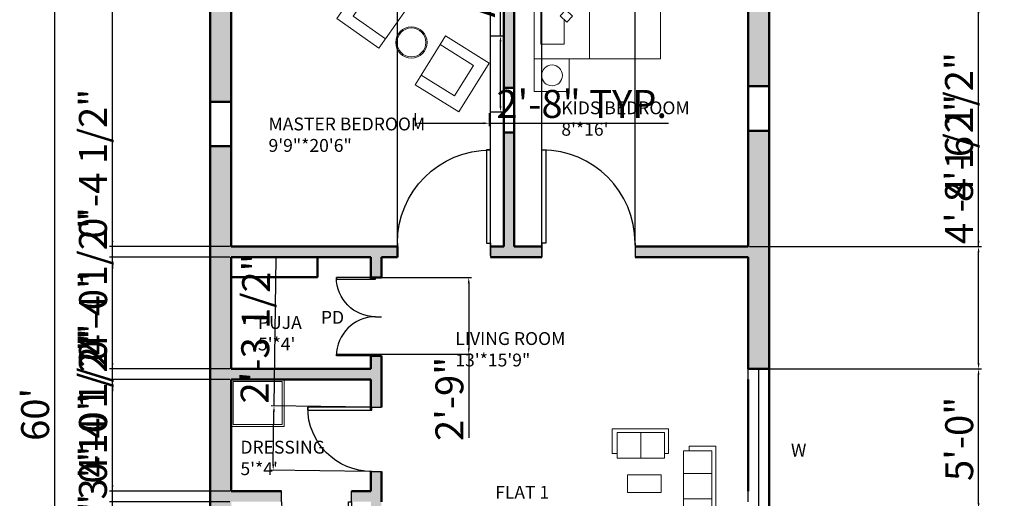
# Model space of a CAD drawing. Units: inches. Extents: x 2063 to 3370, y 2091 to 2971.
# Tile 6 of 14: x 2063 to 2486, y 2468 to 2674. Entities that reach past the tile are written whole.
import ezdxf

# ---------------------------------------------------------------- set-up
doc = ezdxf.new("R2010")
doc.units = ezdxf.units.IN
for name, color, linetype, lineweight in [('A-ANNO-DIMS', 2, 'Continuous', 18), ('A-ANNO-TEXT', 7, 'Continuous', 18), ('A-AREA-IDEN', 3, 'Continuous', 18), ('A-COLS', 7, 'Continuous', 50), ('A-DOOR', 4, 'Continuous', 25), ('A-FURN', 8, 'Continuous', 18), ('A-GLAZ', 131, 'Continuous', 25), ('A-WALL', 7, 'Continuous', 50), ('A-WALL-PATT', 8, 'Continuous', 13)]:
    doc.layers.add(name, color=color, linetype=linetype, lineweight=lineweight)
doc.styles.get("Standard").update_dxf_attribs({"font": 'arial.ttf'})
doc.dimstyles.new('ISO-25', dxfattribs={"dimtxt": 12, "dimasz": 2.5, "dimexe": 1.25, "dimexo": 0.625, "dimtad": 1, "dimdec": 0, "dimlunit": 4, "dimtxsty": 'Standard', "dimcen": 2.5, "dimadec": 0, "dimazin": 0, "dimtfac": 1, "dimtdec": 0, "dimtmove": 0, "dimatfit": 3, "dimfxl": 1, "dimarcsym": 0})

# ---------------------------------------------------------------- blocks, each defined once
blk = doc.blocks.new('*U2')
for p, q in [((0, 0), (0, -6)), ((40, 0), (40, -6))]:
    blk.add_line(p, q)
blk.add_lwpolyline([(0, 0), (0, 40), (1.75, 40), (1.75, 0)], close=True)
blk.add_arc((0, 0), 40, 0, 90)
blk = doc.blocks.new('*D6')
at = {"layer": 'A-ANNO-DIMS', "color": 0, "lineweight": -2, "transparency": 16777216}
for p, q in [((2144.1, 2864.43), (2076.56, 2864.43)), ((2077.81, 2861.93), (2077.81, 2146.93)), ((2144.1, 2144.43), (2076.56, 2144.43))]:
    blk.add_line(p, q, dxfattribs=at)
at = {"layer": 'A-ANNO-DIMS', "color": 0, "transparency": 16777216}
for points in [[(2077.39, 2861.93), (2078.23, 2861.93), (2077.81, 2864.43)], [(2077.39, 2146.93), (2078.23, 2146.93), (2077.81, 2144.43)]]:
    blk.add_solid(points, dxfattribs=at)
at = {"layer": 'Defpoints', "color": 0, "transparency": 16777216}
for p in [(2144.72, 2864.43), (2077.81, 2144.43), (2144.72, 2144.43)]:
    blk.add_point(p, dxfattribs=at)
at = {"layer": 'A-ANNO-DIMS', "color": 0, "transparency": 16777216, "insert": (2071.06, 2504.43), "char_height": 12, "attachment_point": 5, "rotation": 90}
blk.add_mtext("60'", dxfattribs=at)
blk = doc.blocks.new('BED-DOUBLE')
for p, q in [((23.79, 50.98), (30.96, 58.78)), ((30.96, 58.78), (30.96, 50.54)), ((23.79, 14), (23.79, 50.98)), ((30.96, 50.54), (23.79, 50.98))]:
    blk.add_line(p, q)
for points in [[(0, 58.78), (15.11, 58.78), (15.11, 72.78), (0, 72.78)], [(0, 58.78), (54.26, 58.78), (54.26, 14), (0, 14)], [(11.45, 40.86), (13.89, 43.46), (16.84, 40.71), (14.4, 38.1)], [(11.16, 32.43), (13.59, 35.03), (16.54, 32.28), (14.11, 29.67)], [(0, 0), (15.11, 0), (15.11, 14), (0, 14)]]:
    blk.add_lwpolyline(points, close=True)
for points in [[(12.88, 42.39), (12.88, 53.87), (2.9, 53.87), (2.9, 35.71), (12.88, 35.71), (12.88, 39.52)], [(12.88, 34.27), (12.88, 38.39), (2.9, 38.39), (2.9, 20.23), (12.88, 20.23), (12.88, 30.81)]]:
    blk.add_lwpolyline(points)
for centre, radius in [((7.71, 65.74), 4.47), ((15.81, 36.46), 1.81), ((7.71, 6.86), 4.47)]:
    blk.add_circle(centre, radius)
blk = doc.blocks.new('ARMCHAIR')
for p, q in [((10.7, 28.87), (13.03, 32.61)), ((13.03, 32.61), (31.78, 20.96)), ((0, 11.65), (3.54, 17.35)), ((31.78, 20.96), (18.75, 0)), ((18.75, 0), (0, 11.65))]:
    blk.add_line(p, q)
blk.add_lwpolyline([(2.55, 15.75), (16.92, 6.82), (25.07, 19.93), (10.7, 28.87)], close=True)
blk = doc.blocks.new('SOFA-2SEAT')
for p, q in [((0, 2.07), (0, 12.63)), ((0, 12.63), (24.16, 12.63)), ((12.27, 11.03), (12.27, 0)), ((24.16, 12.63), (24.16, 2.07)), ((2.08, 2.07), (0, 2.07)), ((24.16, 2.07), (22.46, 2.07))]:
    blk.add_line(p, q)
blk.add_lwpolyline([(22.46, 0), (2.08, 0), (2.08, 11.03), (22.46, 11.03)], close=True)
blk = doc.blocks.new('SOFA-3SEAT')
for p, q in [((2.4, 33.13), (2.4, 35.12)), ((2.4, 35.12), (13.91, 35.12)), ((13.91, 35.12), (13.91, 0)), ((0, 23.31), (12.18, 23.31)), ((0, 12.42), (12.18, 12.42)), ((2.4, 0), (2.4, 1.81)), ((13.91, 0), (2.4, 0))]:
    blk.add_line(p, q)
blk.add_lwpolyline([(12.18, 33.13), (0, 33.13), (0, 1.81), (12.18, 1.81)], close=True)
blk = doc.blocks.new('*D24')
at = {"layer": 'A-ANNO-DIMS', "color": 0, "lineweight": -2, "transparency": 16777216}
for p, q in [((2269.34, 2666.87), (2269.34, 2866.5)), ((2265.08, 2666.87), (2270.59, 2666.87)), ((2269.34, 2636.76), (2269.34, 2664.37)), ((2265.08, 2634.26), (2270.59, 2634.26))]:
    blk.add_line(p, q, dxfattribs=at)
at = {"layer": 'A-ANNO-DIMS', "color": 0, "transparency": 16777216}
for points in [[(2268.93, 2664.37), (2269.76, 2664.37), (2269.34, 2666.87)], [(2268.93, 2636.76), (2269.76, 2636.76), (2269.34, 2634.26)]]:
    blk.add_solid(points, dxfattribs=at)
at = {"layer": 'Defpoints', "color": 0, "transparency": 16777216}
for p in [(2264.45, 2666.87), (2269.34, 2666.87), (2264.45, 2634.26)]:
    blk.add_point(p, dxfattribs=at)
at = {"layer": 'A-ANNO-DIMS', "color": 0, "transparency": 16777216, "insert": (2262.51, 2767.94), "char_height": 12, "attachment_point": 5, "rotation": 90}
blk.add_mtext('ARMCHAIR 2\'-8 1/2" TYP.', dxfattribs=at)
blk = doc.blocks.new('*D25')
at = {"layer": 'A-ANNO-DIMS', "color": 0, "lineweight": -2, "transparency": 16777216}
for p, q in [((2232.68, 2633.64), (2232.68, 2628.12)), ((2264.45, 2633.64), (2264.45, 2628.12)), ((2235.18, 2629.37), (2261.95, 2629.37)), ((2264.45, 2629.37), (2341.55, 2629.37))]:
    blk.add_line(p, q, dxfattribs=at)
at = {"layer": 'A-ANNO-DIMS', "color": 0, "transparency": 16777216}
for points in [[(2235.18, 2629.79), (2235.18, 2628.95), (2232.68, 2629.37)], [(2261.95, 2629.79), (2261.95, 2628.95), (2264.45, 2629.37)]]:
    blk.add_solid(points, dxfattribs=at)
at = {"layer": 'Defpoints', "color": 0, "transparency": 16777216}
for p in [(2232.68, 2634.26), (2264.45, 2634.26), (2264.45, 2629.37)]:
    blk.add_point(p, dxfattribs=at)
at = {"layer": 'A-ANNO-DIMS', "color": 0, "transparency": 16777216, "insert": (2304.25, 2636.12), "char_height": 12, "attachment_point": 5}
blk.add_mtext('2\'-8" TYP.', dxfattribs=at)
blk = doc.blocks.new('*D50')
at = {"layer": 'A-ANNO-DIMS', "color": 0, "lineweight": -2, "transparency": 16777216}
for p, q in [((2102.72, 2396.38), (2102.72, 2468.18)), ((2153.1, 2396.38), (2101.47, 2396.38)), ((2102.72, 2376.43), (2102.72, 2393.88)), ((2153.1, 2373.93), (2101.47, 2373.93))]:
    blk.add_line(p, q, dxfattribs=at)
at = {"layer": 'A-ANNO-DIMS', "color": 0, "transparency": 16777216}
for points in [[(2102.31, 2393.88), (2103.14, 2393.88), (2102.72, 2396.38)], [(2102.31, 2376.43), (2103.14, 2376.43), (2102.72, 2373.93)]]:
    blk.add_solid(points, dxfattribs=at)
at = {"layer": 'Defpoints', "color": 0, "transparency": 16777216}
for p in [(2102.72, 2396.38), (2153.72, 2396.38), (2153.72, 2373.93)]:
    blk.add_point(p, dxfattribs=at)
at = {"layer": 'A-ANNO-DIMS', "color": 0, "transparency": 16777216, "insert": (2095.89, 2433.53), "char_height": 12, "attachment_point": 5, "rotation": 90}
blk.add_mtext('1\'-10 1/2"', dxfattribs=at)
blk = doc.blocks.new('*D52')
at = {"layer": 'A-ANNO-DIMS', "color": 0, "lineweight": -2, "transparency": 16777216}
for p, q in [((2102.72, 2466.93), (2102.72, 2539.85)), ((2153.1, 2466.93), (2101.47, 2466.93)), ((2102.72, 2422.88), (2102.72, 2464.43)), ((2153.1, 2420.38), (2101.47, 2420.38))]:
    blk.add_line(p, q, dxfattribs=at)
at = {"layer": 'A-ANNO-DIMS', "color": 0, "transparency": 16777216}
for points in [[(2102.31, 2464.43), (2103.14, 2464.43), (2102.72, 2466.93)], [(2102.31, 2422.88), (2103.14, 2422.88), (2102.72, 2420.38)]]:
    blk.add_solid(points, dxfattribs=at)
at = {"layer": 'Defpoints', "color": 0, "transparency": 16777216}
for p in [(2102.72, 2466.93), (2153.72, 2466.93), (2153.72, 2420.38)]:
    blk.add_point(p, dxfattribs=at)
at = {"layer": 'A-ANNO-DIMS', "color": 0, "transparency": 16777216, "insert": (2095.89, 2504.64), "char_height": 12, "attachment_point": 5, "rotation": 90}
blk.add_mtext('3\'-10 1/2"', dxfattribs=at)
blk = doc.blocks.new('*D53')
at = {"layer": 'A-ANNO-DIMS', "color": 0, "lineweight": -2, "transparency": 16777216}
for p, q in [((2102.72, 2473.93), (2102.72, 2537.54)), ((2153.1, 2471.43), (2101.47, 2471.43)), ((2102.72, 2466.93), (2102.72, 2471.43)), ((2153.1, 2466.93), (2101.47, 2466.93)), ((2102.72, 2464.43), (2102.72, 2461.93))]:
    blk.add_line(p, q, dxfattribs=at)
at = {"layer": 'A-ANNO-DIMS', "color": 0, "transparency": 16777216}
for points in [[(2102.31, 2473.93), (2103.14, 2473.93), (2102.72, 2471.43)], [(2102.31, 2464.43), (2103.14, 2464.43), (2102.72, 2466.93)]]:
    blk.add_solid(points, dxfattribs=at)
at = {"layer": 'Defpoints', "color": 0, "transparency": 16777216}
for p in [(2102.72, 2471.43), (2153.72, 2471.43), (2153.72, 2466.93)]:
    blk.add_point(p, dxfattribs=at)
at = {"layer": 'A-ANNO-DIMS', "color": 0, "transparency": 16777216, "insert": (2095.89, 2506.98), "char_height": 12, "attachment_point": 5, "rotation": 90}
blk.add_mtext('0\'-4 1/2"', dxfattribs=at)
blk = doc.blocks.new('*D54')
at = {"layer": 'A-ANNO-DIMS', "color": 0, "lineweight": -2, "transparency": 16777216}
for p, q in [((2153.1, 2519.43), (2101.47, 2519.43)), ((2102.72, 2473.93), (2102.72, 2516.93)), ((2153.1, 2471.43), (2101.47, 2471.43))]:
    blk.add_line(p, q, dxfattribs=at)
at = {"layer": 'A-ANNO-DIMS', "color": 0, "transparency": 16777216}
for points in [[(2102.31, 2516.93), (2103.14, 2516.93), (2102.72, 2519.43)], [(2102.31, 2473.93), (2103.14, 2473.93), (2102.72, 2471.43)]]:
    blk.add_solid(points, dxfattribs=at)
at = {"layer": 'Defpoints', "color": 0, "transparency": 16777216}
for p in [(2102.72, 2519.43), (2153.72, 2519.43), (2153.72, 2471.43)]:
    blk.add_point(p, dxfattribs=at)
at = {"layer": 'A-ANNO-DIMS', "color": 0, "transparency": 16777216, "insert": (2095.97, 2495.43), "char_height": 12, "attachment_point": 5, "rotation": 90}
blk.add_mtext('4\'-0"', dxfattribs=at)
blk = doc.blocks.new('*D55')
at = {"layer": 'A-ANNO-DIMS', "color": 0, "lineweight": -2, "transparency": 16777216}
for p, q in [((2102.72, 2526.43), (2102.72, 2590.04)), ((2153.1, 2523.93), (2101.47, 2523.93)), ((2102.72, 2519.43), (2102.72, 2523.93)), ((2153.1, 2519.43), (2101.47, 2519.43)), ((2102.72, 2516.93), (2102.72, 2514.43))]:
    blk.add_line(p, q, dxfattribs=at)
at = {"layer": 'A-ANNO-DIMS', "color": 0, "transparency": 16777216}
for points in [[(2102.31, 2526.43), (2103.14, 2526.43), (2102.72, 2523.93)], [(2102.31, 2516.93), (2103.14, 2516.93), (2102.72, 2519.43)]]:
    blk.add_solid(points, dxfattribs=at)
at = {"layer": 'Defpoints', "color": 0, "transparency": 16777216}
for p in [(2102.72, 2523.93), (2153.72, 2523.93), (2153.72, 2519.43)]:
    blk.add_point(p, dxfattribs=at)
at = {"layer": 'A-ANNO-DIMS', "color": 0, "transparency": 16777216, "insert": (2095.89, 2559.48), "char_height": 12, "attachment_point": 5, "rotation": 90}
blk.add_mtext('0\'-4 1/2"', dxfattribs=at)
blk = doc.blocks.new('*D56')
at = {"layer": 'A-ANNO-DIMS', "color": 0, "lineweight": -2, "transparency": 16777216}
for p, q in [((2153.1, 2571.93), (2101.47, 2571.93)), ((2102.72, 2526.43), (2102.72, 2569.43)), ((2153.1, 2523.93), (2101.47, 2523.93))]:
    blk.add_line(p, q, dxfattribs=at)
at = {"layer": 'A-ANNO-DIMS', "color": 0, "transparency": 16777216}
for points in [[(2102.31, 2569.43), (2103.14, 2569.43), (2102.72, 2571.93)], [(2102.31, 2526.43), (2103.14, 2526.43), (2102.72, 2523.93)]]:
    blk.add_solid(points, dxfattribs=at)
at = {"layer": 'Defpoints', "color": 0, "transparency": 16777216}
for p in [(2102.72, 2571.93), (2153.72, 2571.93), (2153.72, 2523.93)]:
    blk.add_point(p, dxfattribs=at)
at = {"layer": 'A-ANNO-DIMS', "color": 0, "transparency": 16777216, "insert": (2095.97, 2547.93), "char_height": 12, "attachment_point": 5, "rotation": 90}
blk.add_mtext('4\'-0"', dxfattribs=at)
blk = doc.blocks.new('*D57')
at = {"layer": 'A-ANNO-DIMS', "color": 0, "lineweight": -2, "transparency": 16777216}
for p, q in [((2102.72, 2578.93), (2102.72, 2642.54)), ((2153.1, 2576.43), (2101.47, 2576.43)), ((2102.72, 2571.93), (2102.72, 2576.43)), ((2153.1, 2571.93), (2101.47, 2571.93)), ((2102.72, 2569.43), (2102.72, 2566.93))]:
    blk.add_line(p, q, dxfattribs=at)
at = {"layer": 'A-ANNO-DIMS', "color": 0, "transparency": 16777216}
for points in [[(2102.31, 2578.93), (2103.14, 2578.93), (2102.72, 2576.43)], [(2102.31, 2569.43), (2103.14, 2569.43), (2102.72, 2571.93)]]:
    blk.add_solid(points, dxfattribs=at)
at = {"layer": 'Defpoints', "color": 0, "transparency": 16777216}
for p in [(2102.72, 2576.43), (2153.72, 2576.43), (2153.72, 2571.93)]:
    blk.add_point(p, dxfattribs=at)
at = {"layer": 'A-ANNO-DIMS', "color": 0, "transparency": 16777216, "insert": (2095.89, 2611.98), "char_height": 12, "attachment_point": 5, "rotation": 90}
blk.add_mtext('0\'-4 1/2"', dxfattribs=at)
blk = doc.blocks.new('*D58')
at = {"layer": 'A-ANNO-DIMS', "color": 0, "lineweight": -2, "transparency": 16777216}
for p, q in [((2153.1, 2822.43), (2101.47, 2822.43)), ((2102.72, 2578.93), (2102.72, 2819.93)), ((2153.1, 2576.43), (2101.47, 2576.43))]:
    blk.add_line(p, q, dxfattribs=at)
at = {"layer": 'A-ANNO-DIMS', "color": 0, "transparency": 16777216}
for points in [[(2102.31, 2819.93), (2103.14, 2819.93), (2102.72, 2822.43)], [(2102.31, 2578.93), (2103.14, 2578.93), (2102.72, 2576.43)]]:
    blk.add_solid(points, dxfattribs=at)
at = {"layer": 'Defpoints', "color": 0, "transparency": 16777216}
for p in [(2102.72, 2822.43), (2153.72, 2822.43), (2153.72, 2576.43)]:
    blk.add_point(p, dxfattribs=at)
at = {"layer": 'A-ANNO-DIMS', "color": 0, "transparency": 16777216, "insert": (2095.97, 2699.43), "char_height": 12, "attachment_point": 5, "rotation": 90}
blk.add_mtext('20\'-6"', dxfattribs=at)
blk = doc.blocks.new('*D63')
at = {"layer": 'A-ANNO-DIMS', "color": 0, "lineweight": -2, "transparency": 16777216}
for p, q in [((2376.35, 2523.93), (2475.9, 2523.93)), ((2474.65, 2466.43), (2474.65, 2521.43)), ((2376.35, 2463.93), (2475.9, 2463.93))]:
    blk.add_line(p, q, dxfattribs=at)
at = {"layer": 'A-ANNO-DIMS', "color": 0, "transparency": 16777216}
for points in [[(2474.23, 2521.43), (2475.06, 2521.43), (2474.65, 2523.93)], [(2474.23, 2466.43), (2475.06, 2466.43), (2474.65, 2463.93)]]:
    blk.add_solid(points, dxfattribs=at)
at = {"layer": 'Defpoints', "color": 0, "transparency": 16777216}
for p in [(2375.72, 2523.93), (2474.65, 2523.93), (2375.72, 2463.93)]:
    blk.add_point(p, dxfattribs=at)
at = {"layer": 'A-ANNO-DIMS', "color": 0, "transparency": 16777216, "insert": (2467.89, 2493.93), "char_height": 12, "attachment_point": 5, "rotation": 90}
blk.add_mtext('5\'-0"', dxfattribs=at)
blk = doc.blocks.new('*D64')
at = {"layer": 'A-ANNO-DIMS', "color": 0, "lineweight": -2, "transparency": 16777216}
for p, q in [((2474.65, 2576.43), (2474.65, 2640.52)), ((2376.35, 2576.43), (2475.9, 2576.43)), ((2474.65, 2526.43), (2474.65, 2573.93)), ((2376.35, 2523.93), (2475.9, 2523.93))]:
    blk.add_line(p, q, dxfattribs=at)
at = {"layer": 'A-ANNO-DIMS', "color": 0, "transparency": 16777216}
for points in [[(2474.23, 2573.93), (2475.06, 2573.93), (2474.65, 2576.43)], [(2474.23, 2526.43), (2475.06, 2526.43), (2474.65, 2523.93)]]:
    blk.add_solid(points, dxfattribs=at)
at = {"layer": 'Defpoints', "color": 0, "transparency": 16777216}
for p in [(2375.72, 2576.43), (2474.65, 2576.43), (2375.72, 2523.93)]:
    blk.add_point(p, dxfattribs=at)
at = {"layer": 'A-ANNO-DIMS', "color": 0, "transparency": 16777216, "insert": (2467.82, 2609.72), "char_height": 12, "attachment_point": 5, "rotation": 90}
blk.add_mtext('4\'-4 1/2"', dxfattribs=at)
blk = doc.blocks.new('*D65')
at = {"layer": 'A-ANNO-DIMS', "color": 0, "lineweight": -2, "transparency": 16777216}
for p, q in [((2376.35, 2679.03), (2475.9, 2679.03)), ((2474.65, 2578.93), (2474.65, 2676.53)), ((2376.35, 2576.43), (2475.9, 2576.43))]:
    blk.add_line(p, q, dxfattribs=at)
at = {"layer": 'A-ANNO-DIMS', "color": 0, "transparency": 16777216}
for points in [[(2474.23, 2676.53), (2475.06, 2676.53), (2474.65, 2679.03)], [(2474.23, 2578.93), (2475.06, 2578.93), (2474.65, 2576.43)]]:
    blk.add_solid(points, dxfattribs=at)
at = {"layer": 'Defpoints', "color": 0, "transparency": 16777216}
for p in [(2375.72, 2679.03), (2474.65, 2679.03), (2375.72, 2576.43)]:
    blk.add_point(p, dxfattribs=at)
at = {"layer": 'A-ANNO-DIMS', "color": 0, "transparency": 16777216, "insert": (2467.82, 2627.73), "char_height": 12, "attachment_point": 5, "rotation": 90}
blk.add_mtext('8\'-6 1/2"', dxfattribs=at)
blk = doc.blocks.new('*D72')
at = {"layer": 'A-ANNO-DIMS', "color": 0, "lineweight": -2, "transparency": 16777216}
for p, q in [((2225.08, 2577.05), (2225.08, 2907.68)), ((2227.58, 2906.43), (2262.58, 2906.43)), ((2265.08, 2572.55), (2265.08, 2907.68))]:
    blk.add_line(p, q, dxfattribs=at)
at = {"layer": 'A-ANNO-DIMS', "color": 0, "transparency": 16777216}
for points in [[(2227.58, 2906.84), (2227.58, 2906.01), (2225.08, 2906.43)], [(2262.58, 2906.84), (2262.58, 2906.01), (2265.08, 2906.43)]]:
    blk.add_solid(points, dxfattribs=at)
at = {"layer": 'Defpoints', "color": 0, "transparency": 16777216}
for p in [(2265.08, 2906.43), (2225.08, 2576.43), (2265.08, 2571.93)]:
    blk.add_point(p, dxfattribs=at)
at = {"layer": 'A-ANNO-DIMS', "color": 0, "transparency": 16777216, "insert": (2245.08, 2913.18), "char_height": 12, "attachment_point": 5}
blk.add_mtext('3\'-4"', dxfattribs=at)
blk = doc.blocks.new('*D73')
at = {"layer": 'A-ANNO-DIMS', "color": 0, "lineweight": -2, "transparency": 16777216}
for p, q in [((2287.14, 2572.55), (2287.14, 2907.68)), ((2289.64, 2906.43), (2324.64, 2906.43)), ((2327.14, 2577.05), (2327.14, 2907.68))]:
    blk.add_line(p, q, dxfattribs=at)
at = {"layer": 'A-ANNO-DIMS', "color": 0, "transparency": 16777216}
for points in [[(2289.64, 2906.84), (2289.64, 2906.01), (2287.14, 2906.43)], [(2324.64, 2906.84), (2324.64, 2906.01), (2327.14, 2906.43)]]:
    blk.add_solid(points, dxfattribs=at)
at = {"layer": 'Defpoints', "color": 0, "transparency": 16777216}
for p in [(2327.14, 2906.43), (2327.14, 2576.43), (2287.14, 2571.93)]:
    blk.add_point(p, dxfattribs=at)
at = {"layer": 'A-ANNO-DIMS', "color": 0, "transparency": 16777216, "insert": (2307.14, 2913.18), "char_height": 12, "attachment_point": 5}
blk.add_mtext('3\'-4"', dxfattribs=at)
blk = doc.blocks.new('*D76')
at = {"layer": 'A-ANNO-DIMS', "color": 0, "lineweight": -2, "transparency": 16777216}
for p, q in [((2172.1, 2508.04), (2172.95, 2571.85)), ((2213.47, 2507.48), (2170.85, 2508.06)), ((2171.76, 2483), (2172.06, 2505.54)), ((2213.1, 2479.95), (2170.48, 2480.52))]:
    blk.add_line(p, q, dxfattribs=at)
at = {"layer": 'A-ANNO-DIMS', "color": 0, "transparency": 16777216}
for points in [[(2171.65, 2505.54), (2172.48, 2505.53), (2172.1, 2508.04)], [(2171.34, 2483.01), (2172.18, 2483), (2171.73, 2480.5)]]:
    blk.add_solid(points, dxfattribs=at)
at = {"layer": 'Defpoints', "color": 0, "transparency": 16777216}
for p in [(2172.1, 2508.04), (2214.09, 2507.47), (2213.72, 2479.94)]:
    blk.add_point(p, dxfattribs=at)
at = {"layer": 'A-ANNO-DIMS', "color": 0, "transparency": 16777216, "insert": (2165.71, 2541.28), "char_height": 12, "attachment_point": 5, "rotation": 89.2309}
blk.add_mtext('2\'-3 1/2"', dxfattribs=at)
blk = doc.blocks.new('*D77')
at = {"layer": 'A-ANNO-DIMS', "color": 0, "lineweight": -2, "transparency": 16777216}
for p, q in [((2214.35, 2563.16), (2256.97, 2563.16)), ((2255.72, 2560.66), (2255.72, 2532.76)), ((2214.35, 2530.26), (2256.97, 2530.26)), ((2255.72, 2530.26), (2255.72, 2494.41))]:
    blk.add_line(p, q, dxfattribs=at)
at = {"layer": 'A-ANNO-DIMS', "color": 0, "transparency": 16777216}
for points in [[(2255.31, 2560.66), (2256.14, 2560.66), (2255.72, 2563.16)], [(2255.31, 2532.76), (2256.14, 2532.76), (2255.72, 2530.26)]]:
    blk.add_solid(points, dxfattribs=at)
at = {"layer": 'Defpoints', "color": 0, "transparency": 16777216}
for p in [(2213.72, 2563.16), (2213.72, 2530.26), (2255.72, 2530.26)]:
    blk.add_point(p, dxfattribs=at)
at = {"layer": 'A-ANNO-DIMS', "color": 0, "transparency": 16777216, "insert": (2248.97, 2511.09), "char_height": 12, "attachment_point": 5, "rotation": 90}
blk.add_mtext('2\'-9"', dxfattribs=at)

msp = doc.modelspace()

# ---------------------------------------------------------------- hatches: boundary and pattern name
at = {"layer": 'A-WALL-PATT'}
h = msp.add_hatch(color=256, dxfattribs=at)
h.dxf.hatch_style = 1
h.paths.add_polyline_path([(2275.22, 2822.43), (2270.72, 2822.43), (2270.72, 2815.29), (2275.22, 2815.29)])
h.paths.add_polyline_path([(2384.72, 2777.84), (2375.72, 2777.84), (2375.72, 2774.43), (2371.22, 2774.43), (2275.22, 2774.43), (2275.22, 2777.68), (2270.72, 2777.68), (2270.72, 2644.58), (2275.22, 2644.58), (2275.22, 2769.93), (2375.72, 2769.93), (2375.72, 2727.03), (2384.72, 2727.03)])
h.paths.add_polyline_path([(2384.72, 2812.03), (2375.72, 2812.03), (2375.72, 2801.84), (2384.72, 2801.84)])
h.paths.add_polyline_path([(2275.22, 2625.46), (2270.72, 2625.46), (2270.72, 2576.43), (2265.08, 2576.43), (2265.08, 2571.93), (2287.14, 2571.93), (2287.14, 2576.43), (2275.22, 2576.43)])
h = msp.add_hatch(color=256, dxfattribs=at)
h.dxf.hatch_style = 1
h.paths.add_polyline_path([(2384.72, 2679.03), (2375.72, 2679.03), (2375.72, 2645.28), (2384.72, 2645.28)])
h.paths.add_polyline_path([(2384.72, 2626.16), (2375.72, 2626.16), (2375.72, 2576.43), (2327.14, 2576.43), (2327.14, 2571.93), (2375.72, 2571.93), (2375.72, 2523.93), (2384.72, 2523.93)])
h.paths.add_polyline_path([(2384.72, 2463.93), (2375.72, 2463.93), (2375.72, 2383.04), (2384.72, 2383.04)])
h.paths.add_polyline_path([(2153.72, 2812.31), (2144.72, 2812.31), (2144.72, 2638.63), (2153.72, 2638.63)])
h.paths.add_polyline_path([(2225.08, 2576.43), (2153.72, 2576.43), (2153.72, 2619.52), (2144.72, 2619.52), (2144.72, 2420.38), (2153.72, 2420.38), (2153.72, 2466.93), (2175.31, 2466.93), (2175.31, 2471.43), (2153.72, 2471.43), (2153.72, 2519.43), (2213.72, 2519.43), (2213.72, 2507.47), (2214.09, 2507.47), (2218.22, 2507.47), (2218.22, 2519.43), (2218.22, 2523.93), (2218.22, 2529.53), (2213.72, 2529.53), (2213.72, 2523.93), (2153.72, 2523.93), (2153.72, 2571.93), (2213.72, 2571.93), (2213.72, 2563.16), (2218.22, 2563.16), (2218.22, 2571.93), (2225.08, 2571.93)])
h = msp.add_hatch(color=256, dxfattribs=at)
h.dxf.hatch_style = 1
h.paths.add_polyline_path([(2269.36, 2382.93), (2218.22, 2382.93), (2218.22, 2466.93), (2218.22, 2471.43), (2218.22, 2479.94), (2213.72, 2479.94), (2213.72, 2471.43), (2205.44, 2471.43), (2205.44, 2466.93), (2213.72, 2466.93), (2213.72, 2382.93), (2153.72, 2382.93), (2153.72, 2373.93), (2269.36, 2373.93)])
h.paths.add_polyline_path([(2278.22, 2363.81), (2273.72, 2363.81), (2273.72, 2331.84), (2278.22, 2331.84)])
h.paths.add_polyline_path([(2295.55, 2382.93), (2278.36, 2382.93), (2278.36, 2373.93), (2295.55, 2373.93), (2295.55, 2378.19)])
h.paths.add_polyline_path([(2259.11, 2234.43), (2153.72, 2234.43), (2153.72, 2225.43), (2259.11, 2225.43)])
h.paths.add_polyline_path([(2278.22, 2283.84), (2273.72, 2283.84), (2273.72, 2234.43), (2278.22, 2234.43)])
h.paths.add_polyline_path([(2153.72, 2363.81), (2144.72, 2363.81), (2144.72, 2241.68), (2153.72, 2241.68)])

# ---------------------------------------------------------------- linework, layer by layer
at = {"layer": 'A-COLS'}
msp.add_lwpolyline([(2270.72, 2644.58), (2275.22, 2644.58), (2275.22, 2625.46), (2270.72, 2625.46)], dxfattribs=at)
for points in [[(2375.72, 2645.28), (2384.72, 2645.28), (2384.72, 2626.16), (2375.72, 2626.16)], [(2144.72, 2638.63), (2153.72, 2638.63), (2153.72, 2619.52), (2144.72, 2619.52)]]:
    msp.add_lwpolyline(points, close=True, dxfattribs=at)
at = {"layer": 'A-FURN'}
for points in [[(2153.72, 2519.43), (2176.4, 2519.43), (2176.4, 2499.22), (2153.72, 2499.22)], [(2154.56, 2518.59), (2175.56, 2518.59), (2175.56, 2500.06), (2154.56, 2500.06)], [(2323.84, 2478.46), (2338.31, 2478.46), (2338.31, 2470.9), (2323.84, 2470.9)]]:
    msp.add_lwpolyline(points, close=True, dxfattribs=at)
for radius in [6.72, 6.2]:
    msp.add_circle((2231.09, 2664.05), radius, dxfattribs=at)
at = {"layer": 'A-GLAZ'}
for p, q in [((2375.72, 2466.93), (2375.72, 2523.93)), ((2380.22, 2523.93), (2380.22, 2463.93))]:
    msp.add_line(p, q, dxfattribs=at)
at = {"layer": 'A-WALL'}
for p, q in [((2270.72, 2777.68), (2270.72, 2576.43)), ((2275.22, 2769.93), (2275.22, 2576.43)), ((2153.72, 2576.43), (2225.08, 2576.43)), ((2225.08, 2571.93), (2225.08, 2576.43)), ((2265.08, 2576.43), (2270.72, 2576.43)), ((2275.22, 2576.43), (2287.14, 2576.43)), ((2327.14, 2576.43), (2375.72, 2576.43)), ((2153.72, 2571.93), (2213.72, 2571.93)), ((2153.72, 2571.93), (2213.72, 2571.93)), ((2213.72, 2571.93), (2213.72, 2562.42)), ((2218.22, 2571.93), (2218.22, 2563.16)), ((2218.22, 2571.93), (2225.08, 2571.93)), ((2265.08, 2571.93), (2287.14, 2571.93)), ((2327.14, 2571.93), (2375.72, 2571.93)), ((2213.72, 2563.16), (2218.22, 2563.16)), ((2218.22, 2563.16), (2213.72, 2563.16)), ((2213.72, 2546.46), (2213.72, 2546.23)), ((2213.72, 2530.26), (2213.72, 2523.93)), ((2213.72, 2529.53), (2218.22, 2529.53)), ((2218.22, 2529.53), (2218.22, 2523.93)), ((2153.72, 2523.93), (2213.72, 2523.93)), ((2218.22, 2523.93), (2218.22, 2519.43)), ((2375.72, 2523.93), (2384.72, 2523.93)), ((2153.72, 2519.43), (2213.72, 2519.43)), ((2213.72, 2519.43), (2213.72, 2506.27)), ((2218.22, 2519.43), (2218.22, 2507.47)), ((2213.72, 2479.94), (2213.72, 2471.43)), ((2218.22, 2479.94), (2218.22, 2471.43)), ((2153.72, 2471.43), (2175.31, 2471.43)), ((2205.44, 2471.43), (2213.72, 2471.43)), ((2218.22, 2471.43), (2218.22, 2466.93))]:
    msp.add_line(p, q, dxfattribs=at)
for points in [[(2144.72, 2144.43), (2384.72, 2144.43), (2384.72, 2864.43), (2144.72, 2864.43)], [(2153.72, 2571.93), (2190.7, 2571.93), (2190.7, 2563.33), (2153.72, 2563.33)]]:
    msp.add_lwpolyline(points, close=True, dxfattribs=at)
for points in [[(2153.72, 2822.43), (2153.72, 2576.43)], [(2375.72, 2576.43), (2375.72, 2769.93)], [(2153.72, 2571.93), (2153.72, 2523.93)], [(2375.72, 2523.93), (2375.72, 2571.93)], [(2153.72, 2519.43), (2153.72, 2471.43)], [(2375.72, 2471.43), (2375.72, 2519.43)]]:
    msp.add_lwpolyline(points, dxfattribs=at)

# ---------------------------------------------------------------- block references
at = {"layer": 'A-DOOR', "xscale": -1}
msp.add_blockref('*U2', (2265.08, 2577.93), dxfattribs=at)
at = {"layer": 'A-DOOR'}
msp.add_blockref('*U2', (2287.14, 2577.93), dxfattribs=at)
for p, xscale, yscale, zscale, rotation in [((2215.7, 2563.16), -0.4203428619043682, 0.4203428619043682, 0.4203428619043682, 90), ((2215.7, 2529.53), 0.4203428619043682, 0.4203428619043682, 0.4203428619043682, 90), ((2214.09, 2507.47), -0.6884013341675177, 0.6884013341675177, 0.6884013341675177, 90), ((2205.44, 2466.91), 0.753161428329689, 0.753161428329689, 0.753161428329689, 180)]:
    msp.add_blockref('*U2', p, dxfattribs=dict(at, xscale=xscale, yscale=yscale, zscale=zscale, rotation=rotation))
at = {"layer": 'A-FURN'}
for name, p in [('BED-DOUBLE', (2283.77, 2643.05)), ('ARMCHAIR', (2232.68, 2634.26)), ('SOFA-2SEAT', (2317.31, 2485.65)), ('SOFA-3SEAT', (2347.98, 2455.72))]:
    msp.add_blockref(name, p, dxfattribs=at)
at = {"layer": 'A-FURN', "extrusion": (0, 0, -1), "zscale": -1, "rotation": 66.95512356980241}
msp.add_blockref('ARMCHAIR', (-2206.41, 2657.05), dxfattribs=at)

# ---------------------------------------------------------------- texts
at = {"layer": 'A-ANNO-TEXT', "attachment_point": 1}
for s, heights, insert, char_height in [('PD', [0], (2192.25, 2548.85), 5.523), ('W', [0], (2394.09, 2491.86), 5.52), ('FLAT 1', [14.84], (2267.05, 2473.76), 5.523)]:
    msp.add_mtext_dynamic_manual_height_columns(s, width=106.0361, gutter_width=27.61, heights=heights, dxfattribs=dict(at, insert=insert, char_height=char_height))
at = {"layer": 'A-AREA-IDEN', "attachment_point": 1}
for s, heights, insert, char_height in [("KIDS BEDROOM\\P8'*16'", [0], (2295.49, 2638.75), 5.5229), ('MASTER BEDROOM\\P9\'9"*20\'6"', [0], (2169.74, 2631.82), 5.5229), ("PUJA \\P5'*4'", [14.84], (2165.22, 2546.62), 5.523), ('LIVING ROOM\\P13\'*15\'9"', [0], (2249.96, 2539.74), 5.5229), ("DRESSING\\P5'*4'", [0], (2157.68, 2493.12), 5.523)]:
    msp.add_mtext_dynamic_manual_height_columns(s, width=106.0361, gutter_width=27.61, heights=heights, dxfattribs=dict(at, insert=insert, char_height=char_height))

# ---------------------------------------------------------------- dimensions: what is measured, and where the dimension line sits
at = {"layer": 'A-ANNO-DIMS'}
for base, p1, p2, picture, middle in [((2265.08, 2906.43), (2225.08, 2576.43), (2265.08, 2571.93), '*D72', (2245.08, 2913.18)), ((2327.14, 2906.43), (2287.14, 2571.93), (2327.14, 2576.43), '*D73', (2307.14, 2913.18))]:
    dim = msp.add_linear_dim(base=base, p1=p1, p2=p2, dimstyle='ISO-25', override={"dimdec": 1, "dimlfac": 1, "dimrnd": 0, "dimzin": 1, "dimdsep": 46, "dimlunit": 4, "dimfrac": 2}, dxfattribs=at)
    dim.commit()
    dim.dimension.update_dxf_attribs({"geometry": picture, "text_midpoint": middle})
for base, p1, p2, angle, override, picture, middle in [((2077.81, 2144.43), (2144.72, 2864.43), (2144.72, 2144.43), 90, {"dimclrd": 0, "dimclre": 0, "dimclrt": 0}, '*D6', (2071.06, 2504.43)), ((2102.72, 2822.43), (2153.72, 2576.43), (2153.72, 2822.43), 90, {"dimdec": 1, "dimlfac": 1, "dimrnd": 0, "dimzin": 1, "dimdsep": 46, "dimlunit": 4, "dimfrac": 2}, '*D58', (2095.97, 2699.43)), ((2474.65, 2679.03), (2375.72, 2576.43), (2375.72, 2679.03), 90, {"dimdec": 1, "dimlfac": 1, "dimrnd": 0, "dimzin": 1, "dimdsep": 46, "dimlunit": 4, "dimfrac": 2}, '*D65', (2467.82, 2627.73)), ((2102.72, 2576.43), (2153.72, 2571.93), (2153.72, 2576.43), 90, {"dimdec": 1, "dimlfac": 1, "dimrnd": 0, "dimzin": 1, "dimdsep": 46, "dimlunit": 4, "dimfrac": 2}, '*D57', (2095.89, 2611.98)), ((2474.65, 2576.43), (2375.72, 2523.93), (2375.72, 2576.43), 90, {"dimdec": 1, "dimlfac": 1, "dimrnd": 0, "dimzin": 1, "dimdsep": 46, "dimlunit": 4, "dimfrac": 2}, '*D64', (2467.82, 2609.72)), ((2102.72, 2523.93), (2153.72, 2519.43), (2153.72, 2523.93), 90, {"dimdec": 1, "dimlfac": 1, "dimrnd": 0, "dimzin": 1, "dimdsep": 46, "dimlunit": 4, "dimfrac": 2}, '*D55', (2095.89, 2559.48)), ((2102.72, 2571.93), (2153.72, 2523.93), (2153.72, 2571.93), 90, {"dimdec": 1, "dimlfac": 1, "dimrnd": 0, "dimzin": 1, "dimdsep": 46, "dimlunit": 4, "dimfrac": 2}, '*D56', (2095.97, 2547.93)), ((2172.1, 2508.04), (2213.72, 2479.94), (2214.09, 2507.47), 89.2309, {"dimdec": 1, "dimlfac": 1, "dimrnd": 0, "dimzin": 1, "dimdsep": 46, "dimlunit": 4, "dimfrac": 2}, '*D76', (2165.71, 2541.28)), ((2255.72, 2530.26), (2213.72, 2563.16), (2213.72, 2530.26), 270, {"dimdec": 1, "dimlfac": 1, "dimrnd": 0, "dimzin": 1, "dimdsep": 46, "dimlunit": 4, "dimfrac": 2}, '*D77', (2248.97, 2511.09)), ((2102.722, 2466.9264), (2153.722, 2420.3799), (2153.722, 2466.9264), 90, {"dimdec": 1, "dimlfac": 1, "dimrnd": 0, "dimzin": 1, "dimdsep": 46, "dimlunit": 4, "dimfrac": 2}, '*D52', (2095.8883, 2504.6394)), ((2102.72, 2471.43), (2153.72, 2466.93), (2153.72, 2471.43), 90, {"dimdec": 1, "dimlfac": 1, "dimrnd": 0, "dimzin": 1, "dimdsep": 46, "dimlunit": 4, "dimfrac": 2}, '*D53', (2095.89, 2506.98)), ((2474.65, 2523.93), (2375.72, 2463.93), (2375.72, 2523.93), 90, {"dimdec": 1, "dimlfac": 1, "dimrnd": 0, "dimzin": 1, "dimdsep": 46, "dimlunit": 4, "dimfrac": 2}, '*D63', (2467.89, 2493.93)), ((2102.72, 2519.43), (2153.72, 2471.43), (2153.72, 2519.43), 90, {"dimdec": 1, "dimlfac": 1, "dimrnd": 0, "dimzin": 1, "dimdsep": 46, "dimlunit": 4, "dimfrac": 2}, '*D54', (2095.97, 2495.43)), ((2102.722, 2396.3799), (2153.722, 2373.9264), (2153.722, 2396.3799), 90, {"dimdec": 1, "dimlfac": 1, "dimrnd": 0, "dimzin": 1, "dimdsep": 46, "dimlunit": 4, "dimfrac": 2}, '*D50', (2095.8924, 2433.5321))]:
    dim = msp.add_linear_dim(base=base, p1=p1, p2=p2, angle=angle, dimstyle='ISO-25', override=override, dxfattribs=at)
    dim.commit()
    dim.dimension.update_dxf_attribs({"geometry": picture, "text_midpoint": middle})
dim = msp.add_linear_dim(base=(2269.34, 2666.87), p1=(2264.45, 2634.26), p2=(2264.45, 2666.87), angle=90, text='ARMCHAIR <> TYP.', dimstyle='ISO-25', override={"dimdec": 1, "dimrnd": 0, "dimzin": 1, "dimlunit": 4, "dimfrac": 2}, dxfattribs=at)
dim.commit()
dim.dimension.update_dxf_attribs({"geometry": '*D24', "text_midpoint": (2262.51, 2767.94)})
dim = msp.add_linear_dim(base=(2264.45, 2629.37), p1=(2232.68, 2634.26), p2=(2264.45, 2634.26), text='<> TYP.', dimstyle='ISO-25', override={"dimdec": 1, "dimrnd": 0, "dimzin": 1, "dimlunit": 4, "dimfrac": 2}, dxfattribs=at)
dim.commit()
dim.dimension.update_dxf_attribs({"geometry": '*D25', "text_midpoint": (2304.25, 2636.12)})

doc.saveas('drawing.dxf')
